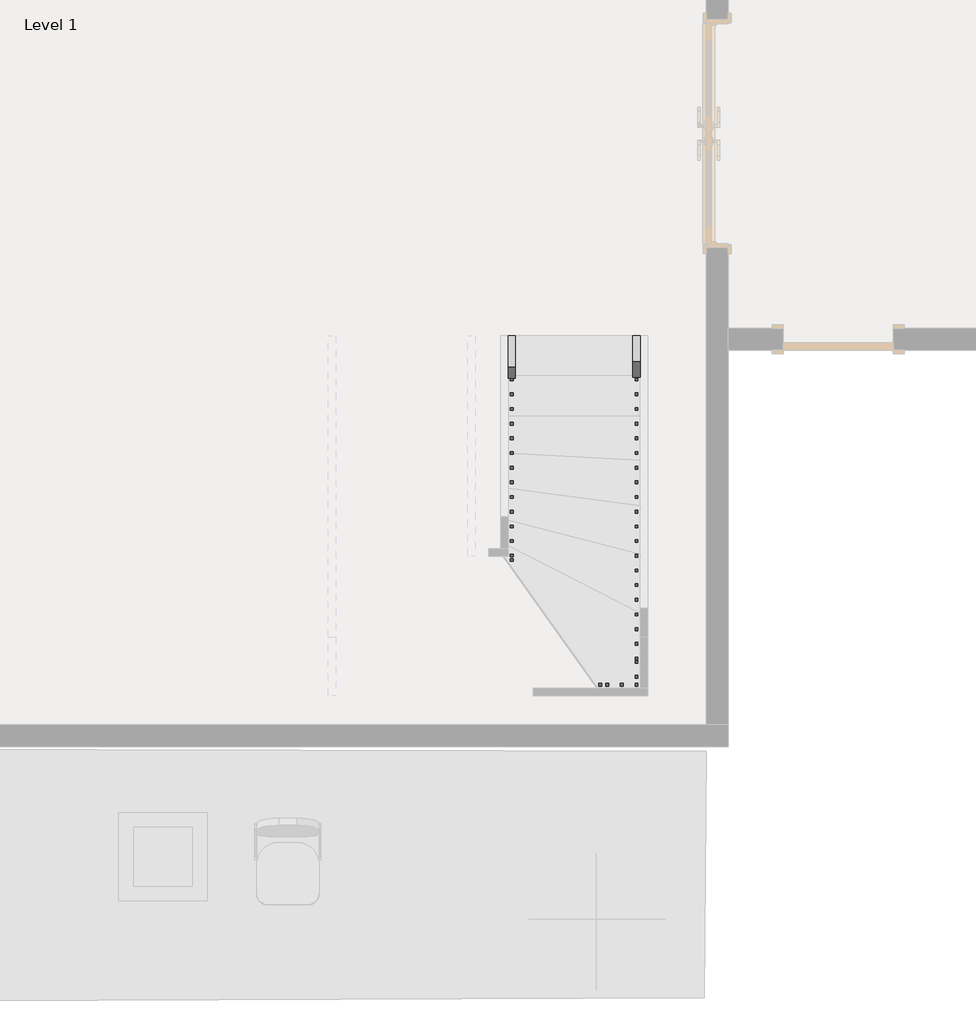
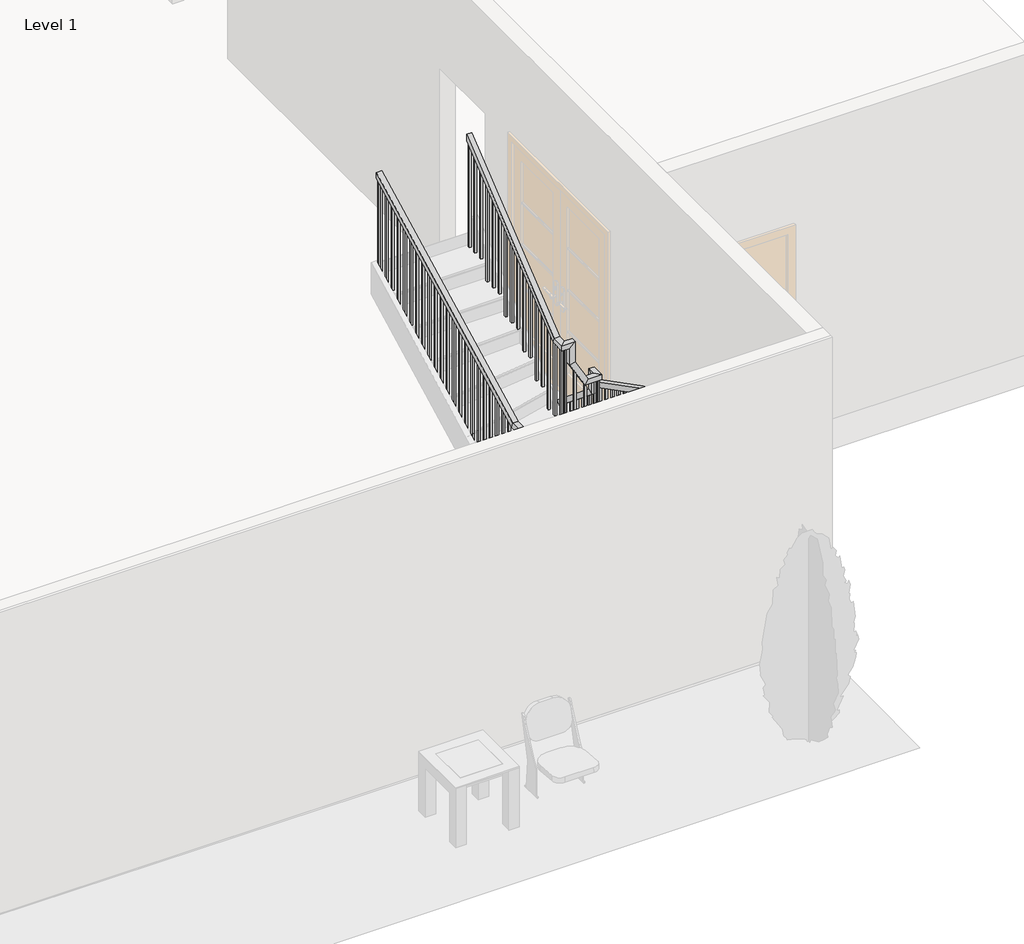
# One storey, part 2 of 3: 2 railings.
"""IFC4 building model written with IfcOpenShell, lengths in millimetres."""

from ifc_helpers import new_model, si_unit, frame, origin, place, context, project, spatial, polyline, outline, extrude, faceted_brep, element, save

model = new_model("IFC4")

# Units and contexts
model_context = context("Model", 3, world=origin())
ifc_project = project(units=[si_unit("LENGTHUNIT", "METRE", prefix="MILLI")], contexts=[model_context])

# Site, building, storey
site = spatial("IfcSite", under=ifc_project)
building = spatial("IfcBuilding", under=site)
storey = spatial("IfcBuildingStorey", under=building, Name="Level 1", Elevation=0.0)

# Railings
placement = place(None, origin())
element("IfcRailing", 1, ObjectType="Handrail - Rectangular", at=placement, inside=storey, context=model_context, shape_type="SolidModel", body=[
    faceted_brep([(-4127.6918623, -2804.4089531, 1025.2529681), (-4127.6918623, -2804.4089531, 959.7067088), (-4178.4918623, -2804.4089531, 959.7067088), (-4178.4918623, -2804.4089531, 1025.2529681), (-4127.6918623, -4255.940645, 2208.7848338), (-4127.6918623, -4306.740645, 2184.659247), (-4178.4918623, -4306.740645, 2184.659247), (-4178.4918623, -4255.940645, 2208.7848338), (-4127.6918623, -4255.940645, 2414.6281882), (-4127.6918623, -4306.740645, 2363.8281882), (-4178.4918623, -4306.740645, 2363.8281882), (-4178.4918623, -4255.940645, 2414.6281882), (-4127.6918623, -4382.940645, 2414.6281882), (-4127.6918623, -4382.940645, 2363.8281882), (-4178.4918623, -4332.140645, 2363.8281882), (-4178.4918623, -4332.140645, 2414.6281882), (-4254.6918623, -4382.940645, 2414.6281882), (-4283.8131962, -4382.940645, 2363.8281882), (-4283.8131962, -4332.140645, 2363.8281882), (-4254.6918623, -4332.140645, 2414.6281882), (-4381.6918623, -4382.940645, 2631.5051451), (-4432.4918623, -4382.940645, 2617.7256424), (-4432.4918623, -4332.140645, 2617.7256424), (-4381.6918623, -4332.140645, 2631.5051451), (-4381.6918623, -4382.940645, 2837.3484995), (-4432.4918623, -4382.940645, 2786.5484995), (-4432.4918623, -4332.140645, 2786.5484995), (-4381.6918623, -4332.140645, 2837.3484995), (-4508.6918623, -4382.940645, 2837.3484995), (-4508.6918623, -4382.940645, 2786.5484995), (-4457.8918623, -4332.140645, 2786.5484995), (-4457.8918623, -4332.140645, 2837.3484995), (-4508.6918623, -4255.940645, 2837.3484995), (-4508.6918623, -4237.8552319, 2786.5484995), (-4457.8918623, -4237.8552319, 2786.5484995), (-4457.8918623, -4255.940645, 2837.3484995), (-4508.6918623, -2804.4089531, 4020.8803652), (-4457.8918623, -2804.4089531, 4020.8803652), (-4457.8918623, -2804.4089531, 3955.3341059), (-4508.6918623, -2804.4089531, 3955.3341059)], [[[0, 1, 2, 3]], [[1, 0, 4, 5]], [[2, 1, 5, 6]], [[3, 2, 6, 7]], [[0, 3, 7, 4]], [[5, 4, 8, 9]], [[6, 5, 9, 10]], [[7, 6, 10, 11]], [[4, 7, 11, 8]], [[9, 8, 12, 13]], [[10, 9, 13, 14]], [[11, 10, 14, 15]], [[8, 11, 15, 12]], [[13, 12, 16, 17]], [[14, 13, 17, 18]], [[15, 14, 18, 19]], [[12, 15, 19, 16]], [[17, 16, 20, 21]], [[18, 17, 21, 22]], [[19, 18, 22, 23]], [[16, 19, 23, 20]], [[21, 20, 24, 25]], [[22, 21, 25, 26]], [[23, 22, 26, 27]], [[20, 23, 27, 24]], [[25, 24, 28, 29]], [[26, 25, 29, 30]], [[27, 26, 30, 31]], [[24, 27, 31, 28]], [[29, 28, 32, 33]], [[30, 29, 33, 34]], [[31, 30, 34, 35]], [[28, 31, 35, 32]], [[36, 37, 38, 39]], [[33, 32, 36, 39]], [[34, 33, 39, 38]], [[35, 34, 38, 37]], [[32, 35, 37, 36]]]),
    extrude(outline(polyline([(-2913.6982886, 3866.2231262), (-2894.6482886, 3881.7558784), (-2894.6482886, 2878.6666667), (-2913.6982886, 2878.6666667), (-2913.6982886, 3866.2231262)])), frame((-4492.8168623, 0.0, 0.0), z_axis=(1.0, 0.0, 0.0), x_axis=(0.0, 1.0, 0.0)), (0.0, 0.0, 1.0), 19.05),
    extrude(outline(polyline([(-3015.2982886, 3783.3817813), (-2996.2482886, 3798.9145334), (-2996.2482886, 2878.6666667), (-3015.2982886, 2878.6666667), (-3015.2982886, 3783.3817813)])), frame((-4492.8168623, 0.0, 0.0), z_axis=(1.0, 0.0, 0.0), x_axis=(0.0, 1.0, 0.0)), (0.0, 0.0, 1.0), 19.05),
    extrude(outline(polyline([(-3116.8982886, 3700.5404364), (-3097.8482886, 3716.0731885), (-3097.8482886, 2709.3333333), (-3116.8982886, 2709.3333333), (-3116.8982886, 3700.5404364)])), frame((-4492.8168623, 0.0, 0.0), z_axis=(1.0, 0.0, 0.0), x_axis=(0.0, 1.0, 0.0)), (0.0, 0.0, 1.0), 19.05),
    extrude(outline(polyline([(-3218.4982886, 3617.6990914), (-3199.4482886, 3633.2318436), (-3199.4482886, 2709.3333333), (-3218.4982886, 2709.3333333), (-3218.4982886, 3617.6990914)])), frame((-4492.8168623, 0.0, 0.0), z_axis=(1.0, 0.0, 0.0), x_axis=(0.0, 1.0, 0.0)), (0.0, 0.0, 1.0), 19.05),
    extrude(outline(polyline([(-3320.0982886, 3534.8577465), (-3301.0482886, 3550.3904987), (-3301.0482886, 2709.3333333), (-3320.0982886, 2709.3333333), (-3320.0982886, 3534.8577465)])), frame((-4492.8168623, 0.0, 0.0), z_axis=(1.0, 0.0, 0.0), x_axis=(0.0, 1.0, 0.0)), (0.0, 0.0, 1.0), 19.05),
    extrude(outline(polyline([(-3421.6982886, 3452.0164016), (-3402.6482886, 3467.5491538), (-3402.6482886, 2540.0), (-3421.6982886, 2540.0), (-3421.6982886, 3452.0164016)])), frame((-4492.8168623, 0.0, 0.0), z_axis=(1.0, 0.0, 0.0), x_axis=(0.0, 1.0, 0.0)), (0.0, 0.0, 1.0), 19.05),
    extrude(outline(polyline([(-3523.2982886, 3369.1750567), (-3504.2482886, 3384.7078088), (-3504.2482886, 2540.0), (-3523.2982886, 2540.0), (-3523.2982886, 3369.1750567)])), frame((-4492.8168623, 0.0, 0.0), z_axis=(1.0, 0.0, 0.0), x_axis=(0.0, 1.0, 0.0)), (0.0, 0.0, 1.0), 19.05),
    extrude(outline(polyline([(-3624.8982886, 3286.3337117), (-3605.8482886, 3301.8664639), (-3605.8482886, 2540.0), (-3624.8982886, 2540.0), (-3624.8982886, 3286.3337117)])), frame((-4492.8168623, 0.0, 0.0), z_axis=(1.0, 0.0, 0.0), x_axis=(0.0, 1.0, 0.0)), (0.0, 0.0, 1.0), 19.05),
    extrude(outline(polyline([(-3726.4982886, 3203.4923668), (-3707.4482886, 3219.025119), (-3707.4482886, 2370.6666667), (-3726.4982886, 2370.6666667), (-3726.4982886, 3203.4923668)])), frame((-4492.8168623, 0.0, 0.0), z_axis=(1.0, 0.0, 0.0), x_axis=(0.0, 1.0, 0.0)), (0.0, 0.0, 1.0), 19.05),
    extrude(outline(polyline([(-3828.0982886, 3120.6510219), (-3809.0482886, 3136.1837741), (-3809.0482886, 2370.6666667), (-3828.0982886, 2370.6666667), (-3828.0982886, 3120.6510219)])), frame((-4492.8168623, 0.0, 0.0), z_axis=(1.0, 0.0, 0.0), x_axis=(0.0, 1.0, 0.0)), (0.0, 0.0, 1.0), 19.05),
    extrude(outline(polyline([(-3929.6982886, 3037.809677), (-3910.6482886, 3053.3424291), (-3910.6482886, 2201.3333333), (-3929.6982886, 2201.3333333), (-3929.6982886, 3037.809677)])), frame((-4492.8168623, 0.0, 0.0), z_axis=(1.0, 0.0, 0.0), x_axis=(0.0, 1.0, 0.0)), (0.0, 0.0, 1.0), 19.05),
    extrude(outline(polyline([(-4031.2982886, 2954.9683321), (-4012.2482886, 2970.5010842), (-4012.2482886, 2201.3333333), (-4031.2982886, 2201.3333333), (-4031.2982886, 2954.9683321)])), frame((-4492.8168623, 0.0, 0.0), z_axis=(1.0, 0.0, 0.0), x_axis=(0.0, 1.0, 0.0)), (0.0, 0.0, 1.0), 19.05),
    extrude(outline(polyline([(-4132.8982886, 2872.1269871), (-4113.8482886, 2887.6597393), (-4113.8482886, 2032.0), (-4132.8982886, 2032.0), (-4132.8982886, 2872.1269871)])), frame((-4492.8168623, 0.0, 0.0), z_axis=(1.0, 0.0, 0.0), x_axis=(0.0, 1.0, 0.0)), (0.0, 0.0, 1.0), 19.05),
    extrude(outline(polyline([(-4234.4982886, 2789.2856422), (-4215.4482886, 2804.8183944), (-4215.4482886, 2032.0), (-4234.4982886, 2032.0), (-4234.4982886, 2789.2856422)])), frame((-4492.8168623, 0.0, 0.0), z_axis=(1.0, 0.0, 0.0), x_axis=(0.0, 1.0, 0.0)), (0.0, 0.0, 1.0), 19.05),
    extrude(outline(polyline([(2496.5834745, -4361.5527661), (2529.115018, -4380.6027661), (1524.0, -4380.6027661), (1524.0, -4361.5527661), (2496.5834745, -4361.5527661)])), frame((0.0, -4367.065645, 0.0), z_axis=(0.0, 1.0, 0.0), x_axis=(0.0, 0.0, 1.0)), (0.0, 0.0, 1.0), 19.05),
    extrude(outline(polyline([(2323.0819089, -4259.9527661), (2355.6134525, -4279.0027661), (1524.0, -4279.0027661), (1524.0, -4259.9527661), (2323.0819089, -4259.9527661)])), frame((0.0, -4367.065645, 0.0), z_axis=(0.0, 1.0, 0.0), x_axis=(0.0, 0.0, 1.0)), (0.0, 0.0, 1.0), 19.05),
    extrude(outline(polyline([(-4236.3339531, 2127.2519138), (-4217.2839531, 2111.7191617), (-4217.2839531, 1016.0), (-4236.3339531, 1016.0), (-4236.3339531, 2127.2519138)])), frame((-4162.6168623, 0.0, 0.0), z_axis=(1.0, 0.0, 0.0), x_axis=(0.0, 1.0, 0.0)), (0.0, 0.0, 1.0), 19.05),
    extrude(outline(polyline([(-4134.7339531, 2044.4105689), (-4115.6839531, 2028.8778167), (-4115.6839531, 1016.0), (-4134.7339531, 1016.0), (-4134.7339531, 2044.4105689)])), frame((-4162.6168623, 0.0, 0.0), z_axis=(1.0, 0.0, 0.0), x_axis=(0.0, 1.0, 0.0)), (0.0, 0.0, 1.0), 19.05),
    extrude(outline(polyline([(-4033.1339531, 1961.569224), (-4014.0839531, 1946.0364718), (-4014.0839531, 846.6666667), (-4033.1339531, 846.6666667), (-4033.1339531, 1961.569224)])), frame((-4162.6168623, 0.0, 0.0), z_axis=(1.0, 0.0, 0.0), x_axis=(0.0, 1.0, 0.0)), (0.0, 0.0, 1.0), 19.05),
    extrude(outline(polyline([(-3931.5339531, 1878.7278791), (-3912.4839531, 1863.1951269), (-3912.4839531, 846.6666667), (-3931.5339531, 846.6666667), (-3931.5339531, 1878.7278791)])), frame((-4162.6168623, 0.0, 0.0), z_axis=(1.0, 0.0, 0.0), x_axis=(0.0, 1.0, 0.0)), (0.0, 0.0, 1.0), 19.05),
    extrude(outline(polyline([(-3829.9339531, 1795.8865341), (-3810.8839531, 1780.353782), (-3810.8839531, 677.3333333), (-3829.9339531, 677.3333333), (-3829.9339531, 1795.8865341)])), frame((-4162.6168623, 0.0, 0.0), z_axis=(1.0, 0.0, 0.0), x_axis=(0.0, 1.0, 0.0)), (0.0, 0.0, 1.0), 19.05),
    extrude(outline(polyline([(-3728.3339531, 1713.0451892), (-3709.2839531, 1697.5124371), (-3709.2839531, 677.3333333), (-3728.3339531, 677.3333333), (-3728.3339531, 1713.0451892)])), frame((-4162.6168623, 0.0, 0.0), z_axis=(1.0, 0.0, 0.0), x_axis=(0.0, 1.0, 0.0)), (0.0, 0.0, 1.0), 19.05),
    extrude(outline(polyline([(-3626.7339531, 1630.2038443), (-3607.6839531, 1614.6710921), (-3607.6839531, 508.0), (-3626.7339531, 508.0), (-3626.7339531, 1630.2038443)])), frame((-4162.6168623, 0.0, 0.0), z_axis=(1.0, 0.0, 0.0), x_axis=(0.0, 1.0, 0.0)), (0.0, 0.0, 1.0), 19.05),
    extrude(outline(polyline([(-3525.1339531, 1547.3624994), (-3506.0839531, 1531.8297472), (-3506.0839531, 508.0), (-3525.1339531, 508.0), (-3525.1339531, 1547.3624994)])), frame((-4162.6168623, 0.0, 0.0), z_axis=(1.0, 0.0, 0.0), x_axis=(0.0, 1.0, 0.0)), (0.0, 0.0, 1.0), 19.05),
    extrude(outline(polyline([(-3423.5339531, 1464.5211545), (-3404.4839531, 1448.9884023), (-3404.4839531, 508.0), (-3423.5339531, 508.0), (-3423.5339531, 1464.5211545)])), frame((-4162.6168623, 0.0, 0.0), z_axis=(1.0, 0.0, 0.0), x_axis=(0.0, 1.0, 0.0)), (0.0, 0.0, 1.0), 19.05),
    extrude(outline(polyline([(-3321.9339531, 1381.6798095), (-3302.8839531, 1366.1470574), (-3302.8839531, 338.6666667), (-3321.9339531, 338.6666667), (-3321.9339531, 1381.6798095)])), frame((-4162.6168623, 0.0, 0.0), z_axis=(1.0, 0.0, 0.0), x_axis=(0.0, 1.0, 0.0)), (0.0, 0.0, 1.0), 19.05),
    extrude(outline(polyline([(-3220.3339531, 1298.8384646), (-3201.2839531, 1283.3057124), (-3201.2839531, 338.6666667), (-3220.3339531, 338.6666667), (-3220.3339531, 1298.8384646)])), frame((-4162.6168623, 0.0, 0.0), z_axis=(1.0, 0.0, 0.0), x_axis=(0.0, 1.0, 0.0)), (0.0, 0.0, 1.0), 19.05),
    extrude(outline(polyline([(-3118.7339531, 1215.9971197), (-3099.6839531, 1200.4643675), (-3099.6839531, 338.6666667), (-3118.7339531, 338.6666667), (-3118.7339531, 1215.9971197)])), frame((-4162.6168623, 0.0, 0.0), z_axis=(1.0, 0.0, 0.0), x_axis=(0.0, 1.0, 0.0)), (0.0, 0.0, 1.0), 19.05),
    extrude(outline(polyline([(-3017.1339531, 1133.1557748), (-2998.0839531, 1117.6230226), (-2998.0839531, 169.3333333), (-3017.1339531, 169.3333333), (-3017.1339531, 1133.1557748)])), frame((-4162.6168623, 0.0, 0.0), z_axis=(1.0, 0.0, 0.0), x_axis=(0.0, 1.0, 0.0)), (0.0, 0.0, 1.0), 19.05),
    extrude(outline(polyline([(-2915.5339531, 1050.3144298), (-2896.4839531, 1034.7816777), (-2896.4839531, 169.3333333), (-2915.5339531, 169.3333333), (-2915.5339531, 1050.3144298)])), frame((-4162.6168623, 0.0, 0.0), z_axis=(1.0, 0.0, 0.0), x_axis=(0.0, 1.0, 0.0)), (0.0, 0.0, 1.0), 19.05),
    extrude(outline(polyline([(-4473.7668623, -4336.0982886), (-4492.8168623, -4336.0982886), (-4492.8168623, -4317.0482886), (-4473.7668623, -4317.0482886), (-4473.7668623, -4336.0982886)])), frame((0.0, 0.0, 1862.6666667), z_axis=(0.0, 0.0, 1.0), x_axis=(1.0, 0.0, 0.0)), (0.0, 0.0, 1.0), 923.8818329),
    extrude(outline(polyline([(-4473.7668623, -4348.015645), (-4473.7668623, -4367.065645), (-4492.8168623, -4367.065645), (-4492.8168623, -4348.015645), (-4473.7668623, -4348.015645)])), frame((0.0, 0.0, 1862.6666667), z_axis=(0.0, 0.0, 1.0), x_axis=(1.0, 0.0, 0.0)), (0.0, 0.0, 1.0), 923.8818329),
    extrude(outline(polyline([(-4458.9809586, -4348.015645), (-4458.9809586, -4367.065645), (-4478.0309586, -4367.065645), (-4478.0309586, -4348.015645), (-4458.9809586, -4348.015645)])), frame((0.0, 0.0, 1693.3333333), z_axis=(0.0, 0.0, 1.0), x_axis=(1.0, 0.0, 0.0)), (0.0, 0.0, 1.0), 1093.2151662),
    extrude(outline(polyline([(-4158.3527661, -4348.015645), (-4158.3527661, -4367.065645), (-4177.4027661, -4367.065645), (-4177.4027661, -4348.015645), (-4158.3527661, -4348.015645)])), frame((0.0, 0.0, 1354.6666667), z_axis=(0.0, 0.0, 1.0), x_axis=(1.0, 0.0, 0.0)), (0.0, 0.0, 1.0), 1009.1615215),
    extrude(outline(polyline([(-4162.6168623, -4348.015645), (-4143.5668623, -4348.015645), (-4143.5668623, -4367.065645), (-4162.6168623, -4367.065645), (-4162.6168623, -4348.015645)])), frame((0.0, 0.0, 1185.3333333), z_axis=(0.0, 0.0, 1.0), x_axis=(1.0, 0.0, 0.0)), (0.0, 0.0, 1.0), 1178.4948549),
    extrude(outline(polyline([(-4162.6168623, -4317.0482886), (-4143.5668623, -4317.0482886), (-4143.5668623, -4336.0982886), (-4162.6168623, -4336.0982886), (-4162.6168623, -4317.0482886)])), frame((0.0, 0.0, 1185.3333333), z_axis=(0.0, 0.0, 1.0), x_axis=(1.0, 0.0, 0.0)), (0.0, 0.0, 1.0), 1178.4948549),
    extrude(outline(polyline([(-2823.4589531, 3939.8013537), (-2804.4089531, 3955.3341059), (-2804.4089531, 2878.6666667), (-2823.4589531, 2878.6666667), (-2823.4589531, 3939.8013537)])), frame((-4492.8168623, 0.0, 0.0), z_axis=(1.0, 0.0, 0.0), x_axis=(0.0, 1.0, 0.0)), (0.0, 0.0, 1.0), 19.05),
    extrude(outline(polyline([(-2823.4589531, 975.239461), (-2804.4089531, 959.7067088), (-2804.4089531, 169.3333333), (-2823.4589531, 169.3333333), (-2823.4589531, 975.239461)])), frame((-4162.6168623, 0.0, 0.0), z_axis=(1.0, 0.0, 0.0), x_axis=(0.0, 1.0, 0.0)), (0.0, 0.0, 1.0), 19.05),
])
element("IfcRailing", 2, ObjectType="Handrail - Rectangular", at=placement, inside=storey, context=model_context, shape_type="SolidModel", body=[
    faceted_brep([(-3264.0918623, -2804.4089531, 1109.0771751), (-3264.0918623, -2804.4089531, 1051.9280057), (-3314.8918623, -2804.4089531, 1051.9280057), (-3314.8918623, -2804.4089531, 1109.0771751), (-3264.0918623, -5064.3908096, 2273.7644996), (-3264.0918623, -5076.7108609, 2222.9644996), (-3314.8918623, -5076.7108609, 2222.9644996), (-3314.8918623, -5064.3908096, 2273.7644996), (-3264.0918623, -5246.540645, 2273.7644996), (-3264.0918623, -5246.540645, 2222.9644996), (-3314.8918623, -5195.740645, 2222.9644996), (-3314.8918623, -5195.740645, 2273.7644996), (-3541.2458149, -5246.540645, 2273.7644996), (-3549.1963911, -5246.540645, 2222.9644996), (-3549.1963911, -5195.740645, 2222.9644996), (-3541.2458149, -5195.740645, 2273.7644996), (-5095.1379097, -5246.540645, 2772.3688337), (-5103.0884858, -5246.540645, 2721.5688337), (-5103.0884858, -5195.740645, 2721.5688337), (-5095.1379097, -5195.740645, 2772.3688337), (-5372.2918623, -5246.540645, 2772.3688337), (-5372.2918623, -5246.540645, 2721.5688337), (-5321.4918623, -5195.740645, 2721.5688337), (-5321.4918623, -5195.740645, 2772.3688337), (-5372.2918623, -5064.3908096, 2772.3688337), (-5372.2918623, -5052.0707583, 2721.5688337), (-5321.4918623, -5052.0707583, 2721.5688337), (-5321.4918623, -5064.3908096, 2772.3688337), (-5372.2918623, -2804.4089531, 3937.0561582), (-5321.4918623, -2804.4089531, 3937.0561582), (-5321.4918623, -2804.4089531, 3879.9069889), (-5372.2918623, -2804.4089531, 3879.9069889)], [[[0, 1, 2, 3]], [[1, 0, 4, 5]], [[2, 1, 5, 6]], [[3, 2, 6, 7]], [[0, 3, 7, 4]], [[5, 4, 8, 9]], [[6, 5, 9, 10]], [[7, 6, 10, 11]], [[4, 7, 11, 8]], [[9, 8, 12, 13]], [[10, 9, 13, 14]], [[11, 10, 14, 15]], [[8, 11, 15, 12]], [[13, 12, 16, 17]], [[14, 13, 17, 18]], [[15, 14, 18, 19]], [[12, 15, 19, 16]], [[17, 16, 20, 21]], [[18, 17, 21, 22]], [[19, 18, 22, 23]], [[16, 19, 23, 20]], [[21, 20, 24, 25]], [[22, 21, 25, 26]], [[23, 22, 26, 27]], [[20, 23, 27, 24]], [[28, 29, 30, 31]], [[25, 24, 28, 31]], [[26, 25, 31, 30]], [[27, 26, 30, 29]], [[24, 27, 29, 28]]]),
    extrude(outline(polyline([(-2819.6658096, 3872.0443296), (-2819.6658096, 2878.6666667), (-2838.7158096, 2878.6666667), (-2838.7158096, 3862.2268642), (-2819.6658096, 3872.0443296)])), frame((-5356.4168623, 0.0, 0.0), z_axis=(1.0, 0.0, 0.0), x_axis=(0.0, 1.0, 0.0)), (0.0, 0.0, 1.0), 19.05),
    extrude(outline(polyline([(-2921.2658096, 3819.6845145), (-2921.2658096, 2878.6666667), (-2940.3158096, 2878.6666667), (-2940.3158096, 3809.8670491), (-2921.2658096, 3819.6845145)])), frame((-5356.4168623, 0.0, 0.0), z_axis=(1.0, 0.0, 0.0), x_axis=(0.0, 1.0, 0.0)), (0.0, 0.0, 1.0), 19.05),
    extrude(outline(polyline([(-3022.8658096, 3767.3246993), (-3022.8658096, 2878.6666667), (-3041.9158096, 2878.6666667), (-3041.9158096, 3757.507234), (-3022.8658096, 3767.3246993)])), frame((-5356.4168623, 0.0, 0.0), z_axis=(1.0, 0.0, 0.0), x_axis=(0.0, 1.0, 0.0)), (0.0, 0.0, 1.0), 19.05),
    extrude(outline(polyline([(-3124.4658096, 3714.9648842), (-3124.4658096, 2709.3333333), (-3143.5158096, 2709.3333333), (-3143.5158096, 3705.1474189), (-3124.4658096, 3714.9648842)])), frame((-5356.4168623, 0.0, 0.0), z_axis=(1.0, 0.0, 0.0), x_axis=(0.0, 1.0, 0.0)), (0.0, 0.0, 1.0), 19.05),
    extrude(outline(polyline([(-3226.0658096, 3662.6050691), (-3226.0658096, 2709.3333333), (-3245.1158096, 2709.3333333), (-3245.1158096, 3652.7876038), (-3226.0658096, 3662.6050691)])), frame((-5356.4168623, 0.0, 0.0), z_axis=(1.0, 0.0, 0.0), x_axis=(0.0, 1.0, 0.0)), (0.0, 0.0, 1.0), 19.05),
    extrude(outline(polyline([(-3327.6658096, 3610.245254), (-3327.6658096, 2709.3333333), (-3346.7158096, 2709.3333333), (-3346.7158096, 3600.4277887), (-3327.6658096, 3610.245254)])), frame((-5356.4168623, 0.0, 0.0), z_axis=(1.0, 0.0, 0.0), x_axis=(0.0, 1.0, 0.0)), (0.0, 0.0, 1.0), 19.05),
    extrude(outline(polyline([(-3429.2658096, 3557.8854389), (-3429.2658096, 2540.0), (-3448.3158096, 2540.0), (-3448.3158096, 3548.0679735), (-3429.2658096, 3557.8854389)])), frame((-5356.4168623, 0.0, 0.0), z_axis=(1.0, 0.0, 0.0), x_axis=(0.0, 1.0, 0.0)), (0.0, 0.0, 1.0), 19.05),
    extrude(outline(polyline([(-3530.8658096, 3505.5256238), (-3530.8658096, 2540.0), (-3549.9158096, 2540.0), (-3549.9158096, 3495.7081584), (-3530.8658096, 3505.5256238)])), frame((-5356.4168623, 0.0, 0.0), z_axis=(1.0, 0.0, 0.0), x_axis=(0.0, 1.0, 0.0)), (0.0, 0.0, 1.0), 19.05),
    extrude(outline(polyline([(-3632.4658096, 3453.1658086), (-3632.4658096, 2540.0), (-3651.5158096, 2540.0), (-3651.5158096, 3443.3483433), (-3632.4658096, 3453.1658086)])), frame((-5356.4168623, 0.0, 0.0), z_axis=(1.0, 0.0, 0.0), x_axis=(0.0, 1.0, 0.0)), (0.0, 0.0, 1.0), 19.05),
    extrude(outline(polyline([(-3734.0658096, 3400.8059935), (-3734.0658096, 2370.6666667), (-3753.1158096, 2370.6666667), (-3753.1158096, 3390.9885282), (-3734.0658096, 3400.8059935)])), frame((-5356.4168623, 0.0, 0.0), z_axis=(1.0, 0.0, 0.0), x_axis=(0.0, 1.0, 0.0)), (0.0, 0.0, 1.0), 19.05),
    extrude(outline(polyline([(-3835.6658096, 3348.4461784), (-3835.6658096, 2370.6666667), (-3854.7158096, 2370.6666667), (-3854.7158096, 3338.6287131), (-3835.6658096, 3348.4461784)])), frame((-5356.4168623, 0.0, 0.0), z_axis=(1.0, 0.0, 0.0), x_axis=(0.0, 1.0, 0.0)), (0.0, 0.0, 1.0), 19.05),
    extrude(outline(polyline([(-3937.2658096, 3296.0863633), (-3937.2658096, 2370.6666667), (-3956.3158096, 2370.6666667), (-3956.3158096, 3286.268898), (-3937.2658096, 3296.0863633)])), frame((-5356.4168623, 0.0, 0.0), z_axis=(1.0, 0.0, 0.0), x_axis=(0.0, 1.0, 0.0)), (0.0, 0.0, 1.0), 19.05),
    extrude(outline(polyline([(-4038.8658096, 3243.7265482), (-4038.8658096, 2201.3333333), (-4057.9158096, 2201.3333333), (-4057.9158096, 3233.9090828), (-4038.8658096, 3243.7265482)])), frame((-5356.4168623, 0.0, 0.0), z_axis=(1.0, 0.0, 0.0), x_axis=(0.0, 1.0, 0.0)), (0.0, 0.0, 1.0), 19.05),
    extrude(outline(polyline([(-4140.4658096, 3191.3667331), (-4140.4658096, 2201.3333333), (-4159.5158096, 2201.3333333), (-4159.5158096, 3181.5492677), (-4140.4658096, 3191.3667331)])), frame((-5356.4168623, 0.0, 0.0), z_axis=(1.0, 0.0, 0.0), x_axis=(0.0, 1.0, 0.0)), (0.0, 0.0, 1.0), 19.05),
    extrude(outline(polyline([(-4242.0658096, 3139.0069179), (-4242.0658096, 2201.3333333), (-4261.1158096, 2201.3333333), (-4261.1158096, 3129.1894526), (-4242.0658096, 3139.0069179)])), frame((-5356.4168623, 0.0, 0.0), z_axis=(1.0, 0.0, 0.0), x_axis=(0.0, 1.0, 0.0)), (0.0, 0.0, 1.0), 19.05),
    extrude(outline(polyline([(-4343.6658096, 3086.6471028), (-4343.6658096, 2032.0), (-4362.7158096, 2032.0), (-4362.7158096, 3076.8296375), (-4343.6658096, 3086.6471028)])), frame((-5356.4168623, 0.0, 0.0), z_axis=(1.0, 0.0, 0.0), x_axis=(0.0, 1.0, 0.0)), (0.0, 0.0, 1.0), 19.05),
    extrude(outline(polyline([(-4445.2658096, 3034.2872877), (-4445.2658096, 2032.0), (-4464.3158096, 2032.0), (-4464.3158096, 3024.4698224), (-4445.2658096, 3034.2872877)])), frame((-5356.4168623, 0.0, 0.0), z_axis=(1.0, 0.0, 0.0), x_axis=(0.0, 1.0, 0.0)), (0.0, 0.0, 1.0), 19.05),
    extrude(outline(polyline([(-4546.8658096, 2981.9274726), (-4546.8658096, 2032.0), (-4565.9158096, 2032.0), (-4565.9158096, 2972.1100073), (-4546.8658096, 2981.9274726)])), frame((-5356.4168623, 0.0, 0.0), z_axis=(1.0, 0.0, 0.0), x_axis=(0.0, 1.0, 0.0)), (0.0, 0.0, 1.0), 19.05),
    extrude(outline(polyline([(-4648.4658096, 2929.5676575), (-4648.4658096, 2032.0), (-4667.5158096, 2032.0), (-4667.5158096, 2919.7501921), (-4648.4658096, 2929.5676575)])), frame((-5356.4168623, 0.0, 0.0), z_axis=(1.0, 0.0, 0.0), x_axis=(0.0, 1.0, 0.0)), (0.0, 0.0, 1.0), 19.05),
    extrude(outline(polyline([(-4750.0658096, 2877.2078424), (-4750.0658096, 1862.6666667), (-4769.1158096, 1862.6666667), (-4769.1158096, 2867.390377), (-4750.0658096, 2877.2078424)])), frame((-5356.4168623, 0.0, 0.0), z_axis=(1.0, 0.0, 0.0), x_axis=(0.0, 1.0, 0.0)), (0.0, 0.0, 1.0), 19.05),
    extrude(outline(polyline([(-4851.6658096, 2824.8480272), (-4851.6658096, 1862.6666667), (-4870.7158096, 1862.6666667), (-4870.7158096, 2815.0305619), (-4851.6658096, 2824.8480272)])), frame((-5356.4168623, 0.0, 0.0), z_axis=(1.0, 0.0, 0.0), x_axis=(0.0, 1.0, 0.0)), (0.0, 0.0, 1.0), 19.05),
    extrude(outline(polyline([(-4953.2658096, 2772.4882121), (-4953.2658096, 1862.6666667), (-4972.3158096, 1862.6666667), (-4972.3158096, 2762.6707468), (-4953.2658096, 2772.4882121)])), frame((-5356.4168623, 0.0, 0.0), z_axis=(1.0, 0.0, 0.0), x_axis=(0.0, 1.0, 0.0)), (0.0, 0.0, 1.0), 19.05),
    extrude(outline(polyline([(-5356.4168623, -5129.065645), (-5356.4168623, -5110.015645), (-5337.3668623, -5110.015645), (-5337.3668623, -5129.065645), (-5356.4168623, -5129.065645)])), frame((0.0, 0.0, 1862.6666667), z_axis=(0.0, 0.0, 1.0), x_axis=(1.0, 0.0, 0.0)), (0.0, 0.0, 1.0), 858.902167),
    extrude(outline(polyline([(-5288.8129097, -5230.665645), (-5307.8629097, -5230.665645), (-5307.8629097, -5211.615645), (-5288.8129097, -5211.615645), (-5288.8129097, -5230.665645)])), frame((0.0, 0.0, 1862.6666667), z_axis=(0.0, 0.0, 1.0), x_axis=(1.0, 0.0, 0.0)), (0.0, 0.0, 1.0), 858.902167),
    extrude(outline(polyline([(-5187.2129097, -5230.665645), (-5206.2629097, -5230.665645), (-5206.2629097, -5211.615645), (-5187.2129097, -5211.615645), (-5187.2129097, -5230.665645)])), frame((0.0, 0.0, 1862.6666667), z_axis=(0.0, 0.0, 1.0), x_axis=(1.0, 0.0, 0.0)), (0.0, 0.0, 1.0), 858.902167),
    extrude(outline(polyline([(2712.4824155, -5074.7708149), (1693.3333333, -5074.7708149), (1693.3333333, -5055.7208149), (2706.3697564, -5055.7208149), (2712.4824155, -5074.7708149)])), frame((0.0, -5230.665645, 0.0), z_axis=(0.0, 1.0, 0.0), x_axis=(0.0, 0.0, 1.0)), (0.0, 0.0, 1.0), 19.05),
    extrude(outline(polyline([(2679.8815673, -4973.1708149), (1693.3333333, -4973.1708149), (1693.3333333, -4954.1208149), (2673.7689082, -4954.1208149), (2679.8815673, -4973.1708149)])), frame((0.0, -5230.665645, 0.0), z_axis=(0.0, 1.0, 0.0), x_axis=(0.0, 0.0, 1.0)), (0.0, 0.0, 1.0), 19.05),
    extrude(outline(polyline([(2647.280719, -4871.5708149), (1693.3333333, -4871.5708149), (1693.3333333, -4852.5208149), (2641.16806, -4852.5208149), (2647.280719, -4871.5708149)])), frame((0.0, -5230.665645, 0.0), z_axis=(0.0, 1.0, 0.0), x_axis=(0.0, 0.0, 1.0)), (0.0, 0.0, 1.0), 19.05),
    extrude(outline(polyline([(2614.6798708, -4769.9708149), (1693.3333333, -4769.9708149), (1693.3333333, -4750.9208149), (2608.5672118, -4750.9208149), (2614.6798708, -4769.9708149)])), frame((0.0, -5230.665645, 0.0), z_axis=(0.0, 1.0, 0.0), x_axis=(0.0, 0.0, 1.0)), (0.0, 0.0, 1.0), 19.05),
    extrude(outline(polyline([(2582.0790226, -4668.3708149), (1693.3333333, -4668.3708149), (1693.3333333, -4649.3208149), (2575.9663635, -4649.3208149), (2582.0790226, -4668.3708149)])), frame((0.0, -5230.665645, 0.0), z_axis=(0.0, 1.0, 0.0), x_axis=(0.0, 0.0, 1.0)), (0.0, 0.0, 1.0), 19.05),
    extrude(outline(polyline([(2549.4781744, -4566.7708149), (1693.3333333, -4566.7708149), (1693.3333333, -4547.7208149), (2543.3655153, -4547.7208149), (2549.4781744, -4566.7708149)])), frame((0.0, -5230.665645, 0.0), z_axis=(0.0, 1.0, 0.0), x_axis=(0.0, 0.0, 1.0)), (0.0, 0.0, 1.0), 19.05),
    extrude(outline(polyline([(2516.8773261, -4465.1708149), (1524.0, -4465.1708149), (1524.0, -4446.1208149), (2510.7646671, -4446.1208149), (2516.8773261, -4465.1708149)])), frame((0.0, -5230.665645, 0.0), z_axis=(0.0, 1.0, 0.0), x_axis=(0.0, 0.0, 1.0)), (0.0, 0.0, 1.0), 19.05),
    extrude(outline(polyline([(2484.2764779, -4363.5708149), (1524.0, -4363.5708149), (1524.0, -4344.5208149), (2478.1638189, -4344.5208149), (2484.2764779, -4363.5708149)])), frame((0.0, -5230.665645, 0.0), z_axis=(0.0, 1.0, 0.0), x_axis=(0.0, 0.0, 1.0)), (0.0, 0.0, 1.0), 19.05),
    extrude(outline(polyline([(2451.6756297, -4261.9708149), (1524.0, -4261.9708149), (1524.0, -4242.9208149), (2445.5629706, -4242.9208149), (2451.6756297, -4261.9708149)])), frame((0.0, -5230.665645, 0.0), z_axis=(0.0, 1.0, 0.0), x_axis=(0.0, 0.0, 1.0)), (0.0, 0.0, 1.0), 19.05),
    extrude(outline(polyline([(2419.0747814, -4160.3708149), (1524.0, -4160.3708149), (1524.0, -4141.3208149), (2412.9621224, -4141.3208149), (2419.0747814, -4160.3708149)])), frame((0.0, -5230.665645, 0.0), z_axis=(0.0, 1.0, 0.0), x_axis=(0.0, 0.0, 1.0)), (0.0, 0.0, 1.0), 19.05),
    extrude(outline(polyline([(2386.4739332, -4058.7708149), (1354.6666667, -4058.7708149), (1354.6666667, -4039.7208149), (2380.3612742, -4039.7208149), (2386.4739332, -4058.7708149)])), frame((0.0, -5230.665645, 0.0), z_axis=(0.0, 1.0, 0.0), x_axis=(0.0, 0.0, 1.0)), (0.0, 0.0, 1.0), 19.05),
    extrude(outline(polyline([(2353.873085, -3957.1708149), (1354.6666667, -3957.1708149), (1354.6666667, -3938.1208149), (2347.7604259, -3938.1208149), (2353.873085, -3957.1708149)])), frame((0.0, -5230.665645, 0.0), z_axis=(0.0, 1.0, 0.0), x_axis=(0.0, 0.0, 1.0)), (0.0, 0.0, 1.0), 19.05),
    extrude(outline(polyline([(2321.2722368, -3855.5708149), (1354.6666667, -3855.5708149), (1354.6666667, -3836.5208149), (2315.1595777, -3836.5208149), (2321.2722368, -3855.5708149)])), frame((0.0, -5230.665645, 0.0), z_axis=(0.0, 1.0, 0.0), x_axis=(0.0, 0.0, 1.0)), (0.0, 0.0, 1.0), 19.05),
    extrude(outline(polyline([(2288.6713885, -3753.9708149), (1354.6666667, -3753.9708149), (1354.6666667, -3734.9208149), (2282.5587295, -3734.9208149), (2288.6713885, -3753.9708149)])), frame((0.0, -5230.665645, 0.0), z_axis=(0.0, 1.0, 0.0), x_axis=(0.0, 0.0, 1.0)), (0.0, 0.0, 1.0), 19.05),
    extrude(outline(polyline([(2256.0705403, -3652.3708149), (1354.6666667, -3652.3708149), (1354.6666667, -3633.3208149), (2249.9578813, -3633.3208149), (2256.0705403, -3652.3708149)])), frame((0.0, -5230.665645, 0.0), z_axis=(0.0, 1.0, 0.0), x_axis=(0.0, 0.0, 1.0)), (0.0, 0.0, 1.0), 19.05),
    extrude(outline(polyline([(-3483.1668623, -5230.665645), (-3502.2168623, -5230.665645), (-3502.2168623, -5211.615645), (-3483.1668623, -5211.615645), (-3483.1668623, -5230.665645)])), frame((0.0, 0.0, 1185.3333333), z_axis=(0.0, 0.0, 1.0), x_axis=(1.0, 0.0, 0.0)), (0.0, 0.0, 1.0), 1037.6311663),
    extrude(outline(polyline([(-3381.5668623, -5230.665645), (-3400.6168623, -5230.665645), (-3400.6168623, -5211.615645), (-3381.5668623, -5211.615645), (-3381.5668623, -5230.665645)])), frame((0.0, 0.0, 1185.3333333), z_axis=(0.0, 0.0, 1.0), x_axis=(1.0, 0.0, 0.0)), (0.0, 0.0, 1.0), 1037.6311663),
    extrude(outline(polyline([(-3279.9668623, -5156.4658096), (-3279.9668623, -5175.5158096), (-3299.0168623, -5175.5158096), (-3299.0168623, -5156.4658096), (-3279.9668623, -5156.4658096)])), frame((0.0, 0.0, 1185.3333333), z_axis=(0.0, 0.0, 1.0), x_axis=(1.0, 0.0, 0.0)), (0.0, 0.0, 1.0), 1037.6311663),
    extrude(outline(polyline([(-5030.0839531, 2198.9352056), (-5030.0839531, 1185.3333333), (-5049.1339531, 1185.3333333), (-5049.1339531, 2208.752671), (-5030.0839531, 2198.9352056)])), frame((-3299.0168623, 0.0, 0.0), z_axis=(1.0, 0.0, 0.0), x_axis=(0.0, 1.0, 0.0)), (0.0, 0.0, 1.0), 19.05),
    extrude(outline(polyline([(-4928.4839531, 2146.5753905), (-4928.4839531, 1185.3333333), (-4947.5339531, 1185.3333333), (-4947.5339531, 2156.3928558), (-4928.4839531, 2146.5753905)])), frame((-3299.0168623, 0.0, 0.0), z_axis=(1.0, 0.0, 0.0), x_axis=(0.0, 1.0, 0.0)), (0.0, 0.0, 1.0), 19.05),
    extrude(outline(polyline([(-4826.8839531, 2094.2155754), (-4826.8839531, 1185.3333333), (-4845.9339531, 1185.3333333), (-4845.9339531, 2104.0330407), (-4826.8839531, 2094.2155754)])), frame((-3299.0168623, 0.0, 0.0), z_axis=(1.0, 0.0, 0.0), x_axis=(0.0, 1.0, 0.0)), (0.0, 0.0, 1.0), 19.05),
    extrude(outline(polyline([(-4725.2839531, 2041.8557603), (-4725.2839531, 1185.3333333), (-4744.3339531, 1185.3333333), (-4744.3339531, 2051.6732256), (-4725.2839531, 2041.8557603)])), frame((-3299.0168623, 0.0, 0.0), z_axis=(1.0, 0.0, 0.0), x_axis=(0.0, 1.0, 0.0)), (0.0, 0.0, 1.0), 19.05),
    extrude(outline(polyline([(-4623.6839531, 1989.4959452), (-4623.6839531, 1016.0), (-4642.7339531, 1016.0), (-4642.7339531, 1999.3134105), (-4623.6839531, 1989.4959452)])), frame((-3299.0168623, 0.0, 0.0), z_axis=(1.0, 0.0, 0.0), x_axis=(0.0, 1.0, 0.0)), (0.0, 0.0, 1.0), 19.05),
    extrude(outline(polyline([(-4522.0839531, 1937.13613), (-4522.0839531, 1016.0), (-4541.1339531, 1016.0), (-4541.1339531, 1946.9535954), (-4522.0839531, 1937.13613)])), frame((-3299.0168623, 0.0, 0.0), z_axis=(1.0, 0.0, 0.0), x_axis=(0.0, 1.0, 0.0)), (0.0, 0.0, 1.0), 19.05),
    extrude(outline(polyline([(-4420.4839531, 1884.7763149), (-4420.4839531, 1016.0), (-4439.5339531, 1016.0), (-4439.5339531, 1894.5937803), (-4420.4839531, 1884.7763149)])), frame((-3299.0168623, 0.0, 0.0), z_axis=(1.0, 0.0, 0.0), x_axis=(0.0, 1.0, 0.0)), (0.0, 0.0, 1.0), 19.05),
    extrude(outline(polyline([(-4318.8839531, 1832.4164998), (-4318.8839531, 1016.0), (-4337.9339531, 1016.0), (-4337.9339531, 1842.2339651), (-4318.8839531, 1832.4164998)])), frame((-3299.0168623, 0.0, 0.0), z_axis=(1.0, 0.0, 0.0), x_axis=(0.0, 1.0, 0.0)), (0.0, 0.0, 1.0), 19.05),
    extrude(outline(polyline([(-4217.2839531, 1780.0566847), (-4217.2839531, 846.6666667), (-4236.3339531, 846.6666667), (-4236.3339531, 1789.87415), (-4217.2839531, 1780.0566847)])), frame((-3299.0168623, 0.0, 0.0), z_axis=(1.0, 0.0, 0.0), x_axis=(0.0, 1.0, 0.0)), (0.0, 0.0, 1.0), 19.05),
    extrude(outline(polyline([(-4115.6839531, 1727.6968696), (-4115.6839531, 846.6666667), (-4134.7339531, 846.6666667), (-4134.7339531, 1737.5143349), (-4115.6839531, 1727.6968696)])), frame((-3299.0168623, 0.0, 0.0), z_axis=(1.0, 0.0, 0.0), x_axis=(0.0, 1.0, 0.0)), (0.0, 0.0, 1.0), 19.05),
    extrude(outline(polyline([(-4014.0839531, 1675.3370545), (-4014.0839531, 846.6666667), (-4033.1339531, 846.6666667), (-4033.1339531, 1685.1545198), (-4014.0839531, 1675.3370545)])), frame((-3299.0168623, 0.0, 0.0), z_axis=(1.0, 0.0, 0.0), x_axis=(0.0, 1.0, 0.0)), (0.0, 0.0, 1.0), 19.05),
    extrude(outline(polyline([(-3912.4839531, 1622.9772393), (-3912.4839531, 677.3333333), (-3931.5339531, 677.3333333), (-3931.5339531, 1632.7947047), (-3912.4839531, 1622.9772393)])), frame((-3299.0168623, 0.0, 0.0), z_axis=(1.0, 0.0, 0.0), x_axis=(0.0, 1.0, 0.0)), (0.0, 0.0, 1.0), 19.05),
    extrude(outline(polyline([(-3810.8839531, 1570.6174242), (-3810.8839531, 677.3333333), (-3829.9339531, 677.3333333), (-3829.9339531, 1580.4348896), (-3810.8839531, 1570.6174242)])), frame((-3299.0168623, 0.0, 0.0), z_axis=(1.0, 0.0, 0.0), x_axis=(0.0, 1.0, 0.0)), (0.0, 0.0, 1.0), 19.05),
    extrude(outline(polyline([(-3709.2839531, 1518.2576091), (-3709.2839531, 677.3333333), (-3728.3339531, 677.3333333), (-3728.3339531, 1528.0750744), (-3709.2839531, 1518.2576091)])), frame((-3299.0168623, 0.0, 0.0), z_axis=(1.0, 0.0, 0.0), x_axis=(0.0, 1.0, 0.0)), (0.0, 0.0, 1.0), 19.05),
    extrude(outline(polyline([(-3607.6839531, 1465.897794), (-3607.6839531, 508.0), (-3626.7339531, 508.0), (-3626.7339531, 1475.7152593), (-3607.6839531, 1465.897794)])), frame((-3299.0168623, 0.0, 0.0), z_axis=(1.0, 0.0, 0.0), x_axis=(0.0, 1.0, 0.0)), (0.0, 0.0, 1.0), 19.05),
    extrude(outline(polyline([(-3506.0839531, 1413.5379789), (-3506.0839531, 508.0), (-3525.1339531, 508.0), (-3525.1339531, 1423.3554442), (-3506.0839531, 1413.5379789)])), frame((-3299.0168623, 0.0, 0.0), z_axis=(1.0, 0.0, 0.0), x_axis=(0.0, 1.0, 0.0)), (0.0, 0.0, 1.0), 19.05),
    extrude(outline(polyline([(-3404.4839531, 1361.1781638), (-3404.4839531, 508.0), (-3423.5339531, 508.0), (-3423.5339531, 1370.9956291), (-3404.4839531, 1361.1781638)])), frame((-3299.0168623, 0.0, 0.0), z_axis=(1.0, 0.0, 0.0), x_axis=(0.0, 1.0, 0.0)), (0.0, 0.0, 1.0), 19.05),
    extrude(outline(polyline([(-3302.8839531, 1308.8183486), (-3302.8839531, 338.6666667), (-3321.9339531, 338.6666667), (-3321.9339531, 1318.635814), (-3302.8839531, 1308.8183486)])), frame((-3299.0168623, 0.0, 0.0), z_axis=(1.0, 0.0, 0.0), x_axis=(0.0, 1.0, 0.0)), (0.0, 0.0, 1.0), 19.05),
    extrude(outline(polyline([(-3201.2839531, 1256.4585335), (-3201.2839531, 338.6666667), (-3220.3339531, 338.6666667), (-3220.3339531, 1266.2759989), (-3201.2839531, 1256.4585335)])), frame((-3299.0168623, 0.0, 0.0), z_axis=(1.0, 0.0, 0.0), x_axis=(0.0, 1.0, 0.0)), (0.0, 0.0, 1.0), 19.05),
    extrude(outline(polyline([(-3099.6839531, 1204.0987184), (-3099.6839531, 338.6666667), (-3118.7339531, 338.6666667), (-3118.7339531, 1213.9161837), (-3099.6839531, 1204.0987184)])), frame((-3299.0168623, 0.0, 0.0), z_axis=(1.0, 0.0, 0.0), x_axis=(0.0, 1.0, 0.0)), (0.0, 0.0, 1.0), 19.05),
    extrude(outline(polyline([(-2998.0839531, 1151.7389033), (-2998.0839531, 169.3333333), (-3017.1339531, 169.3333333), (-3017.1339531, 1161.5563686), (-2998.0839531, 1151.7389033)])), frame((-3299.0168623, 0.0, 0.0), z_axis=(1.0, 0.0, 0.0), x_axis=(0.0, 1.0, 0.0)), (0.0, 0.0, 1.0), 19.05),
    extrude(outline(polyline([(-2896.4839531, 1099.3790882), (-2896.4839531, 169.3333333), (-2915.5339531, 169.3333333), (-2915.5339531, 1109.1965535), (-2896.4839531, 1099.3790882)])), frame((-3299.0168623, 0.0, 0.0), z_axis=(1.0, 0.0, 0.0), x_axis=(0.0, 1.0, 0.0)), (0.0, 0.0, 1.0), 19.05),
    extrude(outline(polyline([(-5356.4168623, -5073.9158096), (-5356.4168623, -5054.8658096), (-5337.3668623, -5054.8658096), (-5337.3668623, -5073.9158096), (-5356.4168623, -5073.9158096)])), frame((0.0, 0.0, 1862.6666667), z_axis=(0.0, 0.0, 1.0), x_axis=(1.0, 0.0, 0.0)), (0.0, 0.0, 1.0), 858.902167),
    extrude(outline(polyline([(-5337.3668623, -5230.665645), (-5356.4168623, -5230.665645), (-5356.4168623, -5211.615645), (-5337.3668623, -5211.615645), (-5337.3668623, -5230.665645)])), frame((0.0, 0.0, 1862.6666667), z_axis=(0.0, 0.0, 1.0), x_axis=(1.0, 0.0, 0.0)), (0.0, 0.0, 1.0), 858.902167),
    extrude(outline(polyline([(2722.0740262, -5104.6629097), (1862.6666667, -5104.6629097), (1862.6666667, -5085.6129097), (2715.9613671, -5085.6129097), (2722.0740262, -5104.6629097)])), frame((0.0, -5230.665645, 0.0), z_axis=(0.0, 1.0, 0.0), x_axis=(0.0, 0.0, 1.0)), (0.0, 0.0, 1.0), 19.05),
    extrude(outline(polyline([(-3531.7208149, -5230.665645), (-3550.7708149, -5230.665645), (-3550.7708149, -5211.615645), (-3531.7208149, -5211.615645), (-3531.7208149, -5230.665645)])), frame((0.0, 0.0, 1185.3333333), z_axis=(0.0, 0.0, 1.0), x_axis=(1.0, 0.0, 0.0)), (0.0, 0.0, 1.0), 1037.6311663),
    extrude(outline(polyline([(-3279.9668623, -5211.615645), (-3279.9668623, -5230.665645), (-3299.0168623, -5230.665645), (-3299.0168623, -5211.615645), (-3279.9668623, -5211.615645)])), frame((0.0, 0.0, 1185.3333333), z_axis=(0.0, 0.0, 1.0), x_axis=(1.0, 0.0, 0.0)), (0.0, 0.0, 1.0), 1037.6311663),
    extrude(outline(polyline([(-5054.8658096, 2211.7065976), (-5054.8658096, 1185.3333333), (-5073.9158096, 1185.3333333), (-5073.9158096, 2221.5240629), (-5054.8658096, 2211.7065976)])), frame((-3299.0168623, 0.0, 0.0), z_axis=(1.0, 0.0, 0.0), x_axis=(0.0, 1.0, 0.0)), (0.0, 0.0, 1.0), 19.05),
    extrude(outline(polyline([(-2804.4089531, 3879.9069889), (-2804.4089531, 2878.6666667), (-2823.4589531, 2878.6666667), (-2823.4589531, 3870.0895235), (-2804.4089531, 3879.9069889)])), frame((-5356.4168623, 0.0, 0.0), z_axis=(1.0, 0.0, 0.0), x_axis=(0.0, 1.0, 0.0)), (0.0, 0.0, 1.0), 19.05),
    extrude(outline(polyline([(-2804.4089531, 1051.9280057), (-2804.4089531, 169.3333333), (-2823.4589531, 169.3333333), (-2823.4589531, 1061.7454711), (-2804.4089531, 1051.9280057)])), frame((-3299.0168623, 0.0, 0.0), z_axis=(1.0, 0.0, 0.0), x_axis=(0.0, 1.0, 0.0)), (0.0, 0.0, 1.0), 19.05),
])

save(model, "model.ifc")

# Revit data of these elements
# Type "Handrail - Rectangular"
#   Assembly Code = "C2010400"
#   built-in parameter 1008612 = 0.0416667 (stored number, unit not read)
#   built-in parameter 1008611 = 0.0416667 (stored number, unit not read)
#   built-in parameter 1008609 = 0.333333 (stored number, unit not read)
#   built-in parameter 1008604 = 0.166667 (stored number, unit not read)
#   built-in parameter 1008603 = 0.166667 (stored number, unit not read)
#   Railing Height = 3' - 0"
#   built-in parameter 1008630 = 2
#   built-in parameter 1008610 = 2
#   built-in parameter 1008618 = Baluster - Square : 3/4"
# Elements 1, 2 (IfcRailing, "Handrail - Rectangular")
#   Phase Created = New Construction
